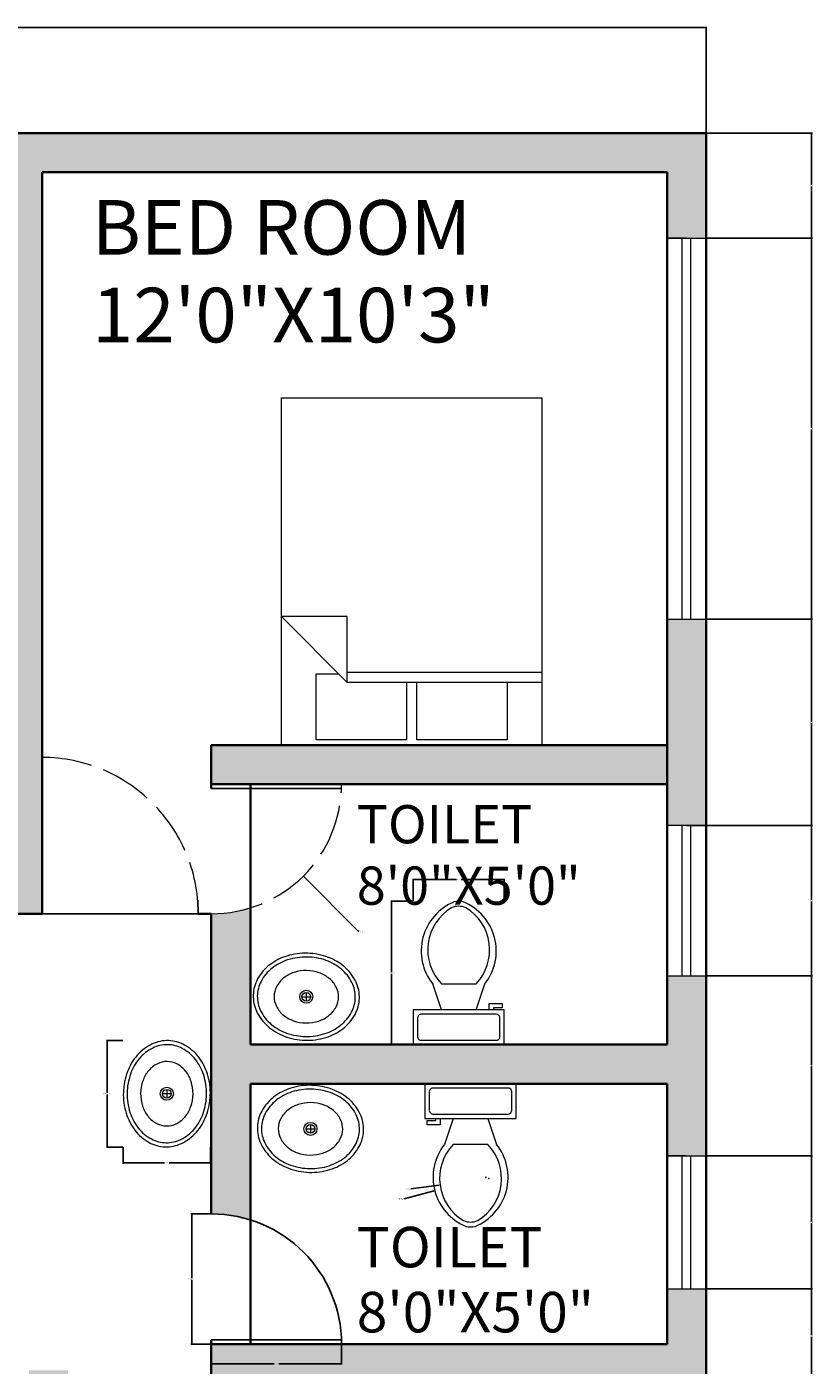
# Model space of a CAD drawing. Units: inches. Extents: x 582 to 1090, y 270 to 781.
# Tile 5 of 5: x 909 to 1090, y 461 to 769. Entities that reach past the tile are written whole.
import ezdxf

# ---------------------------------------------------------------- set-up
doc = ezdxf.new("R2010")
doc.units = ezdxf.units.IN
doc.header["$MEASUREMENT"] = 0
doc.linetypes.add('ACAD_ISO02W100', pattern=[15, 12, -3])
for name, color, linetype, lineweight in [('A-ANNO-DIMS', 2, 'Continuous', 18), ('A-AREA-IDEN', 7, 'Continuous', 25), ('A-DOOR', 3, 'Continuous', 25), ('A-DOOR-SWNG', 3, 'ACAD_ISO02W100', 13), ('A-FLOR-FIXT', 9, 'Continuous', 18), ('A-FURN', 8, 'Continuous', 18), ('A-GLAZ', 4, 'Continuous', 18), ('A-WALL', 7, 'Continuous', 35)]:
    doc.layers.add(name, color=color, linetype=linetype, lineweight=lineweight)
doc.layers.add('A-WALL-PATT', color=9, linetype='Continuous', lineweight=13, true_color=0xc7c8ca)
doc.styles.get("Standard").update_dxf_attribs({"font": 'arial.ttf'})
doc.dimstyles.get("Standard").update_dxf_attribs({"dimtxt": 0.18, "dimasz": 0.18, "dimexe": 0.18, "dimexo": 0.0625, "dimgap": 0.09, "dimtad": 0, "dimtih": 1, "dimtoh": 1, "dimdec": 0, "dimzin": 0, "dimdsep": 46, "dimlunit": 3, "dimtxsty": 'Standard', "dimcen": 0.09, "dimadec": 0, "dimazin": 0, "dimtfac": 1, "dimtdec": 0, "dimtofl": 0, "dimtmove": 0, "dimatfit": 3, "dimfxl": 1, "dimtolj": 1, "dimtzin": 0, "dimarcsym": 0})

# ---------------------------------------------------------------- blocks, each defined once
blk = doc.blocks.new('Toilet - top')
for p, q in [((9.5, -6), (9.5, -2)), ((-10, -8.5), (-8, -8.5)), ((-10, -9.5), (-10, -8.5)), ((-8, -8.5), (-8, -8)), ((-7, -8), (-7, -9.5)), ((-4, -8), (-6, -14)), ((4, -8), (6, -14)), ((-7, -9.5), (-10, -9.5)), ((4, -14), (-4, -14))]:
    blk.add_line(p, q)
blk.add_lwpolyline([(10.5, -8), (10.5, 0), (-10.5, 0), (-10.5, -8)], close=True)
for points in [[(-9.5, -2), (-9.5, -6)], [(8.5, -1), (-8.5, -1)], [(-8.5, -7), (8.5, -7)]]:
    blk.add_lwpolyline(points)
for centre, radius, start, end in [((-8.62, -1.88), 0.884, 81.8699, 188.1301), ((8.62, -1.88), 0.884, 351.8699, 98.1301), ((-8.62, -6.12), 0.884, 171.8699, 278.1301), ((8.62, -6.12), 0.884, 261.8699, 8.1301), ((3.52, -21.58), 12.17, 141.4691, 247.9714), ((4.2, -21.82), 11.33, 136.3677, 238.9468), ((-3.52, -21.58), 12.17, 292.0284, 38.5307), ((-4.2, -21.82), 11.33, 301.053, 43.6321), ((0, -27.88), 4, 245.7318, 294.2682), ((0, -29), 4, 254.8605, 285.1395)]:
    blk.add_arc(centre, radius, start, end)
blk = doc.blocks.new('Sink - Oval top')
for p, q in [((-1, 0), (1, 0)), ((0, 1), (0, -1))]:
    blk.add_line(p, q)
for points in [[(-12.23, 0.39, 0.117634), (-11.46, -3.36, 0.104469), (-8.88, -6.8, 0.090016), (-5.08, -9.07, 0.08192), (-0.32, -10.02, 0.08192), (4.49, -9.38, 0.090016), (8.42, -7.36, 0.104469), (11.22, -4.09, 0.117634), (12.23, -0.39, 0.117634), (11.46, 3.36, 0.104469), (8.88, 6.8, 0.090016), (5.08, 9.07, 0.08192), (0.32, 10.02, 0.08192), (-4.49, 9.38, 0.090016), (-8.42, 7.36, 0.104469), (-11.22, 4.09, 0.117634)], [(-11.29, 0.16, 0.118622), (-10.52, -3.25, 0.104678), (-8.07, -6.36, 0.089562), (-4.54, -8.37, 0.081185), (-0.13, -9.15, 0.081185), (4.3, -8.49, 0.089562), (7.89, -6.58, 0.104678), (10.42, -3.55, 0.118622), (11.29, -0.16, 0.118622), (10.52, 3.25, 0.104678), (8.07, 6.36, 0.089562), (4.54, 8.37, 0.081185), (0.13, 9.15, 0.081185), (-4.3, 8.49, 0.089562), (-7.89, 6.58, 0.104678), (-10.42, 3.55, 0.118622)], [(-7.42, 0.08, 0.118283), (-6.91, -2.17, 0.104607), (-5.29, -4.21, 0.089718), (-2.97, -5.53, 0.081436), (-0.07, -6.04, 0.081436), (2.84, -5.59, 0.089718), (5.2, -4.33, 0.104607), (6.86, -2.32, 0.118283), (7.42, -0.08, 0.118283), (6.91, 2.17, 0.104607), (5.29, 4.21, 0.089718), (2.97, 5.53, 0.081436), (0.07, 6.04, 0.081436), (-2.84, 5.59, 0.089718), (-5.2, 4.33, 0.104607), (-6.86, 2.32, 0.118283)]]:
    blk.add_lwpolyline(points, format="xyb", close=True)
for radius in [1.5, 1]:
    blk.add_circle((0, 0), radius)
blk = doc.blocks.new('Bed - Queen')
for p, q in [((0, -80.00003), (0, 0)), ((0, 0), (59.99999, 0)), ((59.99999, 0), (59.99999, -80.00003)), ((7.99999, -1.2), (28.79998, -1.2)), ((7.99999, -14.4), (7.99999, -1.2)), ((28.79998, -1.2), (28.79998, -14.4)), ((31.19999, -1.2), (51.99999, -1.2)), ((31.19999, -14.4), (31.19999, -1.2)), ((51.99999, -1.2), (51.99999, -16.4)), ((0, -14.4), (44.8, -14.4)), ((59.99999, -29.6), (44.8, -14.4)), ((44.8, -14.4), (44.8, -29.6)), ((44.8, -16.8), (0, -16.8)), ((51.99999, -16.4), (46.79936, -16.4)), ((44.8, -29.6), (59.99999, -29.6)), ((59.99999, -80.00003), (0, -80.00003))]:
    blk.add_line(p, q)
blk = doc.blocks.new('DOOR-SINGLE-30IN')
for p, q in [((29, 0), (29, 30)), ((30, 0), (30, 30))]:
    blk.add_line(p, q)
blk.add_arc((30, 0), 30, 90, 180)
blk = doc.blocks.new('*D12')
at = {"layer": 'A-ANNO-DIMS', "color": 0, "lineweight": -2, "transparency": 16777216}
for p, q in [((931.42, 535.41), (927.62, 535.41)), ((927.8, 535.23), (927.8, 523.32)), ((927.8, 511.04), (927.8, 522.96)), ((931.42, 510.86), (927.62, 510.86))]:
    blk.add_line(p, q, dxfattribs=at)
at = {"layer": 'A-ANNO-DIMS', "color": 0, "transparency": 16777216}
for points in [[(927.77, 535.23), (927.83, 535.23), (927.8, 535.41)], [(927.77, 511.04), (927.83, 511.04), (927.8, 510.86)]]:
    blk.add_solid(points, dxfattribs=at)
at = {"layer": 'Defpoints', "color": 0, "transparency": 16777216}
for p in [(931.49, 535.41), (927.8, 510.86), (931.49, 510.86)]:
    blk.add_point(p, dxfattribs=at)
at = {"layer": 'A-ANNO-DIMS', "color": 0, "transparency": 16777216, "insert": (927.8, 523.14), "char_height": 0.18, "attachment_point": 5}
blk.add_mtext('\\A1;BASIN 25 TYP.', dxfattribs=at)
blk = doc.blocks.new('*D13')
at = {"layer": 'A-ANNO-DIMS', "color": 0, "lineweight": -2, "transparency": 16777216}
for p, q in [((931.49, 510.8), (931.49, 507)), ((951.62, 510.8), (951.62, 507)), ((931.67, 507.18), (941.03, 507.18)), ((951.44, 507.18), (942.08, 507.18))]:
    blk.add_line(p, q, dxfattribs=at)
at = {"layer": 'A-ANNO-DIMS', "color": 0, "transparency": 16777216}
for points in [[(931.67, 507.21), (931.67, 507.15), (931.49, 507.18)], [(951.44, 507.21), (951.44, 507.15), (951.62, 507.18)]]:
    blk.add_solid(points, dxfattribs=at)
at = {"layer": 'Defpoints', "color": 0, "transparency": 16777216}
for p in [(931.49, 510.86), (951.62, 510.86), (951.62, 507.18)]:
    blk.add_point(p, dxfattribs=at)
at = {"layer": 'A-ANNO-DIMS', "color": 0, "transparency": 16777216, "insert": (941.56, 507.18), "char_height": 0.18, "attachment_point": 5}
blk.add_mtext('\\A1;20 TYP.', dxfattribs=at)
blk = doc.blocks.new('*D14')
at = {"layer": 'A-ANNO-DIMS', "color": 0, "lineweight": -2, "transparency": 16777216}
for p, q in [((998.24, 567.49), (993.17, 567.49)), ((993.35, 567.31), (993.35, 551.15)), ((993.35, 534.63), (993.35, 550.79)), ((998.24, 534.45), (993.17, 534.45))]:
    blk.add_line(p, q, dxfattribs=at)
at = {"layer": 'A-ANNO-DIMS', "color": 0, "transparency": 16777216}
for points in [[(993.32, 567.31), (993.38, 567.31), (993.35, 567.49)], [(993.32, 534.63), (993.38, 534.63), (993.35, 534.45)]]:
    blk.add_solid(points, dxfattribs=at)
at = {"layer": 'Defpoints', "color": 0, "transparency": 16777216}
for p in [(998.3, 567.49), (993.35, 534.45), (998.3, 534.45)]:
    blk.add_point(p, dxfattribs=at)
at = {"layer": 'A-ANNO-DIMS', "color": 0, "transparency": 16777216, "insert": (993.35, 550.97), "char_height": 0.18, "attachment_point": 5}
blk.add_mtext('\\A1;WC 33 TYP.', dxfattribs=at)
blk = doc.blocks.new('*D15')
at = {"layer": 'A-ANNO-DIMS', "color": 0, "lineweight": -2, "transparency": 16777216}
for p, q in [((998.3, 567.55), (998.3, 572.63)), ((998.48, 572.45), (1008.28, 572.45)), ((1019.12, 572.45), (1009.33, 572.45)), ((1019.3, 567.55), (1019.3, 572.63))]:
    blk.add_line(p, q, dxfattribs=at)
at = {"layer": 'A-ANNO-DIMS', "color": 0, "transparency": 16777216}
for points in [[(998.48, 572.48), (998.48, 572.42), (998.3, 572.45)], [(1019.12, 572.48), (1019.12, 572.42), (1019.3, 572.45)]]:
    blk.add_solid(points, dxfattribs=at)
at = {"layer": 'Defpoints', "color": 0, "transparency": 16777216}
for p in [(998.3, 572.45), (998.3, 567.49), (1019.3, 567.49)]:
    blk.add_point(p, dxfattribs=at)
at = {"layer": 'A-ANNO-DIMS', "color": 0, "transparency": 16777216, "insert": (1008.8, 572.45), "char_height": 0.18, "attachment_point": 5}
blk.add_mtext('\\A1;21 TYP.', dxfattribs=at)
blk = doc.blocks.new('*D28')
at = {"layer": 'A-ANNO-DIMS', "color": 0, "lineweight": -2, "transparency": 16777216}
for p, q in [((951.74, 495.45), (947.12, 495.45)), ((947.3, 495.27), (947.3, 480.63)), ((947.3, 465.63), (947.3, 480.26)), ((951.74, 465.45), (947.12, 465.45))]:
    blk.add_line(p, q, dxfattribs=at)
at = {"layer": 'A-ANNO-DIMS', "color": 0, "transparency": 16777216}
for points in [[(947.27, 495.27), (947.33, 495.27), (947.3, 495.45)], [(947.27, 465.63), (947.33, 465.63), (947.3, 465.45)]]:
    blk.add_solid(points, dxfattribs=at)
at = {"layer": 'Defpoints', "color": 0, "transparency": 16777216}
for p in [(951.8, 495.45), (947.3, 465.45), (951.8, 465.45)]:
    blk.add_point(p, dxfattribs=at)
at = {"layer": 'A-ANNO-DIMS', "color": 0, "transparency": 16777216, "insert": (947.3, 480.45), "char_height": 0.18, "attachment_point": 5}
blk.add_mtext('\\A1;DOOR 30 TYP.', dxfattribs=at)
blk = doc.blocks.new('*D29')
at = {"layer": 'A-ANNO-DIMS', "color": 0, "lineweight": -2, "transparency": 16777216}
for p, q in [((951.8, 465.38), (951.8, 460.77)), ((981.8, 465.38), (981.8, 460.77)), ((951.98, 460.95), (966.28, 460.95)), ((981.62, 460.95), (967.33, 460.95))]:
    blk.add_line(p, q, dxfattribs=at)
at = {"layer": 'A-ANNO-DIMS', "color": 0, "transparency": 16777216}
for points in [[(951.98, 460.98), (951.98, 460.92), (951.8, 460.95)], [(981.62, 460.98), (981.62, 460.92), (981.8, 460.95)]]:
    blk.add_solid(points, dxfattribs=at)
at = {"layer": 'Defpoints', "color": 0, "transparency": 16777216}
for p in [(951.8, 465.45), (981.8, 465.45), (981.8, 460.95)]:
    blk.add_point(p, dxfattribs=at)
at = {"layer": 'A-ANNO-DIMS', "color": 0, "transparency": 16777216, "insert": (966.8, 460.95), "char_height": 0.18, "attachment_point": 5}
blk.add_mtext('\\A1;30 TYP.', dxfattribs=at)
blk = doc.blocks.new('*D34')
at = {"layer": 'A-ANNO-DIMS', "color": 0, "lineweight": -2, "transparency": 16777216}
for p, q in [((606.8, 744.51), (606.8, 768.93)), ((606.98, 768.75), (836.01, 768.75)), ((1065.62, 768.75), (836.6, 768.75)), ((1065.8, 744.51), (1065.8, 768.93))]:
    blk.add_line(p, q, dxfattribs=at)
at = {"layer": 'A-ANNO-DIMS', "color": 0, "transparency": 16777216}
for points in [[(606.98, 768.78), (606.98, 768.72), (606.8, 768.75)], [(1065.62, 768.78), (1065.62, 768.72), (1065.8, 768.75)]]:
    blk.add_solid(points, dxfattribs=at)
at = {"layer": 'Defpoints', "color": 0, "transparency": 16777216}
for p in [(1065.8, 768.75), (606.8, 744.45), (1065.8, 744.45)]:
    blk.add_point(p, dxfattribs=at)
at = {"layer": 'A-ANNO-DIMS', "color": 0, "transparency": 16777216, "insert": (836.3, 768.75), "char_height": 0.18, "attachment_point": 5}
blk.add_mtext('\\A1;459', dxfattribs=at)
blk = doc.blocks.new('*D52')
at = {"layer": 'A-ANNO-DIMS', "color": 0, "lineweight": -2, "transparency": 16777216}
for p, q in [((1065.87, 744.45), (1090.28, 744.45)), ((1090.1, 744.27), (1090.1, 732.52)), ((1090.1, 720.42), (1090.1, 732.16)), ((1065.87, 720.24), (1090.28, 720.24))]:
    blk.add_line(p, q, dxfattribs=at)
at = {"layer": 'A-ANNO-DIMS', "color": 0, "transparency": 16777216}
for points in [[(1090.07, 744.27), (1090.13, 744.27), (1090.1, 744.45)], [(1090.07, 720.42), (1090.13, 720.42), (1090.1, 720.24)]]:
    blk.add_solid(points, dxfattribs=at)
at = {"layer": 'Defpoints', "color": 0, "transparency": 16777216}
for p in [(1065.8, 744.45), (1090.1, 744.45), (1065.8, 720.24)]:
    blk.add_point(p, dxfattribs=at)
at = {"layer": 'A-ANNO-DIMS', "color": 0, "transparency": 16777216, "insert": (1090.1, 732.34), "char_height": 0.18, "attachment_point": 5}
blk.add_mtext('\\A1;24.21', dxfattribs=at)
blk = doc.blocks.new('*D53')
at = {"layer": 'A-ANNO-DIMS', "color": 0, "lineweight": -2, "transparency": 16777216}
for p, q in [((1065.87, 720.24), (1090.28, 720.24)), ((1090.1, 720.06), (1090.1, 676.52)), ((1090.1, 632.62), (1090.1, 676.16)), ((1065.87, 632.44), (1090.28, 632.44))]:
    blk.add_line(p, q, dxfattribs=at)
at = {"layer": 'A-ANNO-DIMS', "color": 0, "transparency": 16777216}
for points in [[(1090.07, 720.06), (1090.13, 720.06), (1090.1, 720.24)], [(1090.07, 632.62), (1090.13, 632.62), (1090.1, 632.44)]]:
    blk.add_solid(points, dxfattribs=at)
at = {"layer": 'Defpoints', "color": 0, "transparency": 16777216}
for p in [(1065.8, 720.24), (1090.1, 720.24), (1065.8, 632.44)]:
    blk.add_point(p, dxfattribs=at)
at = {"layer": 'A-ANNO-DIMS', "color": 0, "transparency": 16777216, "insert": (1090.1, 676.34), "char_height": 0.18, "attachment_point": 5}
blk.add_mtext('\\A1;87.8', dxfattribs=at)
blk = doc.blocks.new('*D54')
at = {"layer": 'A-ANNO-DIMS', "color": 0, "lineweight": -2, "transparency": 16777216}
for p, q in [((1065.87, 632.44), (1090.28, 632.44)), ((1090.1, 632.26), (1090.1, 608.87)), ((1090.1, 585.11), (1090.1, 608.5)), ((1065.87, 584.93), (1090.28, 584.93))]:
    blk.add_line(p, q, dxfattribs=at)
at = {"layer": 'A-ANNO-DIMS', "color": 0, "transparency": 16777216}
for points in [[(1090.07, 632.26), (1090.13, 632.26), (1090.1, 632.44)], [(1090.07, 585.11), (1090.13, 585.11), (1090.1, 584.93)]]:
    blk.add_solid(points, dxfattribs=at)
at = {"layer": 'Defpoints', "color": 0, "transparency": 16777216}
for p in [(1065.8, 632.44), (1090.1, 632.44), (1065.8, 584.93)]:
    blk.add_point(p, dxfattribs=at)
at = {"layer": 'A-ANNO-DIMS', "color": 0, "transparency": 16777216, "insert": (1090.1, 608.69), "char_height": 0.18, "attachment_point": 5}
blk.add_mtext('\\A1;47.5', dxfattribs=at)
blk = doc.blocks.new('*D55')
at = {"layer": 'A-ANNO-DIMS', "color": 0, "lineweight": -2, "transparency": 16777216}
for p, q in [((1065.87, 584.93), (1090.28, 584.93)), ((1090.1, 584.75), (1090.1, 567.78)), ((1090.1, 550.44), (1090.1, 567.41)), ((1065.87, 550.26), (1090.28, 550.26))]:
    blk.add_line(p, q, dxfattribs=at)
at = {"layer": 'A-ANNO-DIMS', "color": 0, "transparency": 16777216}
for points in [[(1090.07, 584.75), (1090.13, 584.75), (1090.1, 584.93)], [(1090.07, 550.44), (1090.13, 550.44), (1090.1, 550.26)]]:
    blk.add_solid(points, dxfattribs=at)
at = {"layer": 'Defpoints', "color": 0, "transparency": 16777216}
for p in [(1065.8, 584.93), (1090.1, 584.93), (1065.8, 550.26)]:
    blk.add_point(p, dxfattribs=at)
at = {"layer": 'A-ANNO-DIMS', "color": 0, "transparency": 16777216, "insert": (1090.1, 567.6), "char_height": 0.18, "attachment_point": 5}
blk.add_mtext('\\A1;34.675', dxfattribs=at)
blk = doc.blocks.new('*D56')
at = {"layer": 'A-ANNO-DIMS', "color": 0, "lineweight": -2, "transparency": 16777216}
for p, q in [((1065.87, 550.26), (1090.28, 550.26)), ((1090.1, 550.08), (1090.1, 529.74)), ((1090.1, 509.04), (1090.1, 529.38)), ((1065.87, 508.86), (1090.28, 508.86))]:
    blk.add_line(p, q, dxfattribs=at)
at = {"layer": 'A-ANNO-DIMS', "color": 0, "transparency": 16777216}
for points in [[(1090.07, 550.08), (1090.13, 550.08), (1090.1, 550.26)], [(1090.07, 509.04), (1090.13, 509.04), (1090.1, 508.86)]]:
    blk.add_solid(points, dxfattribs=at)
at = {"layer": 'Defpoints', "color": 0, "transparency": 16777216}
for p in [(1065.8, 550.26), (1090.1, 550.26), (1065.8, 508.86)]:
    blk.add_point(p, dxfattribs=at)
at = {"layer": 'A-ANNO-DIMS', "color": 0, "transparency": 16777216, "insert": (1090.1, 529.56), "char_height": 0.18, "attachment_point": 5}
blk.add_mtext('\\A1;41.4', dxfattribs=at)
blk = doc.blocks.new('*D57')
at = {"layer": 'A-ANNO-DIMS', "color": 0, "lineweight": -2, "transparency": 16777216}
for p, q in [((1065.87, 508.86), (1090.28, 508.86)), ((1090.1, 508.68), (1090.1, 493.72)), ((1090.1, 478.39), (1090.1, 493.35)), ((1065.87, 478.21), (1090.28, 478.21))]:
    blk.add_line(p, q, dxfattribs=at)
at = {"layer": 'A-ANNO-DIMS', "color": 0, "transparency": 16777216}
for points in [[(1090.07, 508.68), (1090.13, 508.68), (1090.1, 508.86)], [(1090.07, 478.39), (1090.13, 478.39), (1090.1, 478.21)]]:
    blk.add_solid(points, dxfattribs=at)
at = {"layer": 'Defpoints', "color": 0, "transparency": 16777216}
for p in [(1065.8, 508.86), (1090.1, 508.86), (1065.8, 478.21)]:
    blk.add_point(p, dxfattribs=at)
at = {"layer": 'A-ANNO-DIMS', "color": 0, "transparency": 16777216, "insert": (1090.1, 493.54), "char_height": 0.18, "attachment_point": 5}
blk.add_mtext('\\A1;30.64', dxfattribs=at)
blk = doc.blocks.new('*D58')
at = {"layer": 'A-ANNO-DIMS', "color": 0, "lineweight": -2, "transparency": 16777216}
for p, q in [((1065.87, 478.21), (1090.28, 478.21)), ((1090.1, 478.03), (1090.1, 467.51)), ((1090.1, 456.63), (1090.1, 467.15)), ((1056.87, 456.45), (1090.28, 456.45))]:
    blk.add_line(p, q, dxfattribs=at)
at = {"layer": 'A-ANNO-DIMS', "color": 0, "transparency": 16777216}
for points in [[(1090.07, 478.03), (1090.13, 478.03), (1090.1, 478.21)], [(1090.07, 456.63), (1090.13, 456.63), (1090.1, 456.45)]]:
    blk.add_solid(points, dxfattribs=at)
at = {"layer": 'Defpoints', "color": 0, "transparency": 16777216}
for p in [(1065.8, 478.21), (1090.1, 478.21), (1056.8, 456.45)]:
    blk.add_point(p, dxfattribs=at)
at = {"layer": 'A-ANNO-DIMS', "color": 0, "transparency": 16777216, "insert": (1090.1, 467.33), "char_height": 0.18, "attachment_point": 5}
blk.add_mtext('\\A1;21.77', dxfattribs=at)
blk = doc.blocks.new('*D68')
at = {"layer": 'A-ANNO-DIMS', "color": 0, "lineweight": -2, "transparency": 16777216}
for p, q in [((951.88, 594.45), (952.06, 594.45)), ((951.97, 594.36), (951.97, 594.54)), ((985.63, 560.6), (973.14, 573.16)), ((985.81, 560.6), (985.63, 560.6))]:
    blk.add_line(p, q, dxfattribs=at)
at = {"layer": 'A-ANNO-DIMS', "color": 0, "transparency": 16777216}
blk.add_solid([(973.16, 573.18), (973.11, 573.14), (973.01, 573.29)], dxfattribs=at)
at = {"layer": 'Defpoints', "color": 0, "transparency": 16777216}
for p in [(951.97, 594.45), (973.01, 573.29)]:
    blk.add_point(p, dxfattribs=at)
at = {"layer": 'A-ANNO-DIMS', "color": 0, "transparency": 16777216, "insert": (986.29, 560.6), "char_height": 0.18, "attachment_point": 5}
blk.add_mtext('\\A1;R29.84', dxfattribs=at)
blk = doc.blocks.new('*D78')
at = {"layer": 'A-ANNO-DIMS', "color": 0, "lineweight": -2, "transparency": 16777216}
for p, q in [((1014.96, 503.87), (1015.14, 503.87)), ((1015.05, 503.78), (1015.05, 503.96)), ((996.22, 498.92), (1003.11, 500.73))]:
    blk.add_line(p, q, dxfattribs=at)
at = {"layer": 'A-ANNO-DIMS', "color": 0, "transparency": 16777216}
blk.add_solid([(1003.1, 500.76), (1003.11, 500.7), (1003.28, 500.77)], dxfattribs=at)
at = {"layer": 'Defpoints', "color": 0, "transparency": 16777216}
for p in [(1015.05, 503.87), (1003.28, 500.77)]:
    blk.add_point(p, dxfattribs=at)
at = {"layer": 'A-ANNO-DIMS', "color": 0, "transparency": 16777216, "insert": (995.54, 498.92), "char_height": 0.18, "attachment_point": 5}
blk.add_mtext('\\A1;6X R12.17', dxfattribs=at)
blk = doc.blocks.new('*D79')
at = {"layer": 'A-ANNO-DIMS', "color": 0, "lineweight": -2, "transparency": 16777216}
for p, q in [((1015.64, 503.63), (1015.82, 503.63)), ((1015.73, 503.54), (1015.73, 503.72)), ((997.76, 501.21), (1004.32, 502.1))]:
    blk.add_line(p, q, dxfattribs=at)
at = {"layer": 'A-ANNO-DIMS', "color": 0, "transparency": 16777216}
blk.add_solid([(1004.32, 502.12), (1004.33, 502.07), (1004.5, 502.12)], dxfattribs=at)
at = {"layer": 'Defpoints', "color": 0, "transparency": 16777216}
for p in [(1015.73, 503.63), (1004.5, 502.12)]:
    blk.add_point(p, dxfattribs=at)
at = {"layer": 'A-ANNO-DIMS', "color": 0, "transparency": 16777216, "insert": (997.09, 501.21), "char_height": 0.18, "attachment_point": 5}
blk.add_mtext('\\A1;6X R11.33', dxfattribs=at)

msp = doc.modelspace()

# ---------------------------------------------------------------- hatches: boundary and pattern name
at = {"layer": 'A-WALL-PATT'}
h = msp.add_hatch(color=256, dxfattribs=at)
h.dxf.hatch_style = 1
h.paths.add_polyline_path([(867.8047, 744.446), (765.8047, 744.446), (606.8047, 744.446), (606.8047, 711.9379), (615.8047, 711.9379), (615.8047, 735.446), (756.8047, 735.446), (756.8047, 585.446), (765.8047, 585.446), (765.8047, 735.446), (868.9478, 735.446, -0.06325422)])
h.paths.add_polyline_path([(1065.8047, 744.446), (912.8047, 744.446), (903.8047, 744.446), (903.8047, 708.446), (903.8047, 594.446), (903.8047, 564.6071), (912.8047, 564.6071), (912.8047, 600.6071), (912.8047, 735.446), (1056.8047, 735.446), (1056.8047, 720.2375), (1065.8047, 720.2375)])
h.paths.add_polyline_path([(1065.8047, 632.4383), (1056.8047, 632.4383), (1056.8047, 594.446), (1056.8047, 584.9343), (1065.8047, 584.9343), (1065.8047, 594.446)], flags=17)
h.paths.add_polyline_path([(1056.8047, 603.446), (951.8047, 603.446), (951.8047, 594.446), (1056.8047, 594.446)], flags=17)
h.paths.add_polyline_path([(1065.8047, 525.446), (1065.8047, 550.2593), (1056.8047, 550.2593), (1056.8047, 534.446), (960.8047, 534.446), (960.8047, 565.946, -0.07397332), (952.1262, 564.6071), (951.8047, 564.6071), (951.8047, 495.446, -0.07632083), (960.8047, 494.0641), (960.8047, 525.446), (1056.8047, 525.446), (1056.8047, 508.8565), (1065.8047, 508.8565)])
h.paths.add_polyline_path([(1065.8047, 478.2143), (1056.8047, 478.2143), (1056.8047, 465.446), (951.8047, 465.446), (951.8047, 456.446), (1056.8047, 456.446), (1056.8047, 420.446), (1065.8047, 420.446), (1065.8047, 456.446)])
h.paths.add_polyline_path([(1065.8047, 420.446), (1056.8047, 420.446), (1017.8047, 420.446), (1017.8047, 456.446), (1008.8047, 456.446), (1008.8047, 411.446), (1038.8047, 411.446), (1065.8047, 411.446)])
h.paths.add_polyline_path([(1065.8047, 411.446), (1056.8047, 411.446), (1056.8047, 327.446), (1065.8047, 327.446)])
h.paths.add_polyline_path([(1065.8047, 327.446), (1056.8047, 327.446), (1017.8047, 327.446), (1017.8047, 382.8278, -0.07632083), (1008.8047, 381.446), (1008.8047, 327.446), (983.7348, 327.446), (983.7348, 318.446), (1065.8047, 318.446)])
h.paths.add_polyline_path([(946.9624, 327.446), (918.8047, 327.446), (918.8047, 369.8742), (918.8047, 459.446), (909.8047, 459.446), (909.8047, 369.8742), (909.8047, 318.446), (946.9624, 318.446)])
h.paths.add_polyline_path([(918.8047, 318.446), (909.8047, 318.446), (909.8047, 303.4372), (765.8047, 303.4372), (765.8047, 327.446), (756.8047, 327.446), (756.8047, 294.4372), (918.8047, 294.4372)])
h.paths.add_polyline_path([(909.8047, 378.8742), (882.3477, 378.8742), (882.3477, 347.0959), (889.3299, 347.0959), (889.3299, 369.8742), (909.8047, 369.8742)])
h.paths.add_polyline_path([(779.4225, 378.8742), (765.8047, 378.8742), (765.8047, 369.8742), (779.4225, 369.8742)])
h.paths.add_polyline_path([(765.8047, 516.446), (756.8047, 516.446), (756.8047, 480.446), (756.8047, 336.446), (724.1731, 336.446), (724.1731, 327.446), (765.8047, 327.446), (765.8047, 369.8742), (765.8047, 378.8742)])
h.paths.add_polyline_path([(615.8047, 516.446), (606.8047, 516.446), (606.8047, 327.446), (637.062, 327.446), (637.062, 336.446), (615.8047, 336.446)])
h.paths.add_polyline_path([(615.8047, 631.6498), (606.8047, 631.6498), (606.8047, 585.446), (606.8047, 569.338), (615.8047, 569.338), (615.8047, 585.446), (615.8047, 594.446)])
h.paths.add_polyline_path([(721.9478, 594.446), (615.8047, 594.446), (615.8047, 585.446), (627.9505, 585.446, -0.03261849), (629.8936, 585.446), (710.8047, 585.446), (710.8047, 525.446), (675.3033, 525.446), (675.3033, 516.446), (719.8047, 516.446), (720.8047, 516.446), (720.8047, 525.446), (719.8047, 525.446), (719.8047, 585.446), (720.8047, 585.446, -0.06325422)])
h.paths.add_polyline_path([(646.6852, 525.446), (615.8047, 525.446), (615.8047, 516.446), (645.3033, 516.446, -0.07632083)])
h.paths.add_polyline_path([(615.8047, 525.446), (615.8047, 539.7667), (606.8047, 539.7667), (606.8047, 516.446), (615.8047, 516.446)])

# ---------------------------------------------------------------- linework, layer by layer
at = {"layer": 'A-DOOR'}
for p, q in [((912.8047, 564.6071), (912.8047, 600.6071)), ((951.8047, 594.446), (981.8047, 594.446)), ((951.8047, 594.446), (951.8047, 593.446)), ((951.8047, 593.446), (951.8047, 594.446)), ((951.8047, 593.446), (981.8047, 593.446)), ((948.8047, 564.6071), (948.6663, 567.7605)), ((912.8047, 564.6071), (948.8047, 564.6071)), ((951.8047, 465.446), (951.8047, 466.446))]:
    msp.add_line(p, q, dxfattribs=at)
at = {"layer": 'A-DOOR-SWNG'}
for centre, radius, start, end in [((912.8047, 564.6071), 36, 0, 90), ((951.9654, 594.446), 29.8393, 269.691354, 0)]:
    msp.add_arc(centre, radius, start, end, dxfattribs=at)
at = {"layer": 'A-GLAZ'}
for p, q in [((1061.3047, 720.2375), (1056.8047, 720.2375)), ((1056.8047, 720.2375), (1065.8047, 720.2375)), ((1060.3047, 632.4383), (1060.3047, 720.2375)), ((1062.3047, 632.4383), (1062.3047, 720.2375)), ((1056.8047, 632.4383), (1065.8047, 632.4383)), ((1065.8047, 584.9343), (1056.8047, 584.9343)), ((1060.3047, 550.2593), (1060.3047, 584.9343)), ((1061.3047, 584.9343), (1065.8047, 584.9343)), ((1062.3047, 550.2593), (1062.3047, 584.9343)), ((1056.8047, 550.2593), (1065.8047, 550.2593)), ((1061.3047, 508.8565), (1056.8047, 508.8565)), ((1056.8047, 508.8565), (1065.8047, 508.8565)), ((1060.3047, 478.2143), (1060.3047, 508.8565)), ((1062.3047, 478.2143), (1062.3047, 508.8565)), ((1056.8047, 478.2143), (1065.8047, 478.2143))]:
    msp.add_line(p, q, dxfattribs=at)
at = {"layer": 'A-WALL'}
for p, q in [((912.8047, 744.446), (765.8047, 744.446)), ((1065.8047, 744.446), (912.8047, 744.446)), ((1065.8047, 594.446), (1065.8047, 744.446)), ((912.8047, 594.446), (912.8047, 735.446)), ((912.8047, 735.446), (1056.8047, 735.446)), ((1056.8047, 735.446), (1056.8047, 594.446)), ((951.8047, 603.446), (1056.8047, 603.446)), ((951.8047, 593.446), (951.8047, 603.446)), ((912.8047, 564.6071), (912.8047, 594.446)), ((951.8047, 594.446), (1056.8047, 594.446)), ((960.8047, 534.446), (960.8047, 594.446)), ((1056.8047, 594.446), (1056.8047, 534.446)), ((1065.8047, 594.446), (1065.8047, 318.446)), ((903.8047, 564.6071), (912.8047, 564.6071)), ((951.8047, 564.6071), (948.8047, 564.6071)), ((951.8047, 534.446), (951.8047, 564.6071)), ((951.8047, 495.446), (951.8047, 564.6071)), ((1056.8047, 534.446), (960.8047, 534.446)), ((1056.8047, 525.446), (960.8047, 525.446)), ((960.8047, 465.446), (960.8047, 525.446)), ((1056.8047, 525.446), (1056.8047, 465.446)), ((1065.8047, 525.446), (1065.8047, 465.446)), ((951.8047, 456.446), (951.8047, 466.446)), ((1056.8047, 465.446), (951.8047, 465.446))]:
    msp.add_line(p, q, dxfattribs=at)

# ---------------------------------------------------------------- block references
at = {"layer": 'A-DOOR', "rotation": 269.9999999999998}
msp.add_blockref('DOOR-SINGLE-30IN', (951.8047, 495.4463), dxfattribs=at)
at = {"layer": 'A-FLOR-FIXT'}
for name, p, rotation in [('Toilet - top', (1008.8047, 534.446), 180), ('Sink - Oval top', (941.5552, 523.1387), 270)]:
    msp.add_blockref(name, p, dxfattribs=dict(at, rotation=rotation))
for name, p in [('Sink - Oval top', (973.693, 545.4778)), ('Sink - Oval top', (974.6475, 515.0452)), ('Toilet - top', (1011.5297, 525.446))]:
    msp.add_blockref(name, p, dxfattribs=at)
at = {"layer": 'A-FURN', "rotation": 180}
msp.add_blockref('Bed - Queen', (1027.9385, 603.446), dxfattribs=at)

# ---------------------------------------------------------------- texts
at = {"layer": 'A-ANNO-DIMS'}
for s, height, p in [('12\'0"X10\'3"', 12.580749, (924.3048, 696.216)), ('8\'0"X5\'0"', 8.80313, (985.3127, 566.675)), ('8\'0"X5\'0"', 9.32307, (985.3127, 468.1654))]:
    msp.add_text(s, height=height, dxfattribs=at).set_placement(p)
at = {"layer": 'A-AREA-IDEN'}
for s, height, p in [('BED ROOM', 12.58075, (924.3048, 716.4258)), ('TOILET', 8.80313, (985.3127, 580.8165)), ('TOILET', 9.32307, (985.3127, 483.1421))]:
    msp.add_text(s, height=height, dxfattribs=at).set_placement(p)

# ---------------------------------------------------------------- dimensions: what is measured, and where the dimension line sits
at = {"layer": 'A-ANNO-DIMS'}
dim = msp.add_linear_dim(base=(1065.8047, 768.746), p1=(606.8047, 744.446), p2=(1065.8047, 744.446), dimstyle='Standard', override={"dimdec": 0, "dimlfac": 1, "dimrnd": 0, "dimzin": 0, "dimdsep": 46, "dimlunit": 2}, dxfattribs=at)
dim.commit()
dim.dimension.update_dxf_attribs({"geometry": '*D34', "text_midpoint": (836.3047, 768.746)})
for base, p1, p2, override, picture, middle in [((1090.1047, 744.446), (1065.8047, 720.2375), (1065.8047, 744.446), {"dimdec": 2, "dimlfac": 1, "dimrnd": 0, "dimzin": 0, "dimdsep": 46, "dimlunit": 2}, '*D52', (1090.1047, 732.3417)), ((1090.1047, 720.2375), (1065.8047, 632.4383), (1065.8047, 720.2375), {"dimdec": 1, "dimlfac": 1, "dimrnd": 0, "dimzin": 0, "dimdsep": 46, "dimlunit": 2}, '*D53', (1090.1047, 676.3379)), ((1090.1047, 632.4383), (1065.8047, 584.9343), (1065.8047, 632.4383), {"dimdec": 1, "dimlfac": 1, "dimrnd": 0, "dimzin": 0, "dimdsep": 46, "dimlunit": 2}, '*D54', (1090.1047, 608.6863)), ((1090.1047, 584.9343), (1065.8047, 550.2593), (1065.8047, 584.9343), {"dimdec": 3, "dimlfac": 1, "dimrnd": 0, "dimzin": 0, "dimdsep": 46, "dimlunit": 2}, '*D55', (1090.1047, 567.5968)), ((1090.1047, 550.2593), (1065.8047, 508.8565), (1065.8047, 550.2593), {"dimdec": 1, "dimlfac": 1, "dimrnd": 0, "dimzin": 0, "dimdsep": 46, "dimlunit": 2}, '*D56', (1090.1047, 529.5579)), ((1090.1047, 508.8565), (1065.8047, 478.2143), (1065.8047, 508.8565), {"dimdec": 2, "dimlfac": 1, "dimrnd": 0, "dimzin": 0, "dimdsep": 46, "dimlunit": 2}, '*D57', (1090.1047, 493.5354)), ((1090.1047, 478.2143), (1056.8047, 456.446), (1065.8047, 478.2143), {"dimdec": 2, "dimlfac": 1, "dimrnd": 0, "dimzin": 0, "dimdsep": 46, "dimlunit": 2}, '*D58', (1090.1047, 467.3301))]:
    dim = msp.add_linear_dim(base=base, p1=p1, p2=p2, angle=90, dimstyle='Standard', override=override, dxfattribs=at)
    dim.commit()
    dim.dimension.update_dxf_attribs({"geometry": picture, "text_midpoint": middle})
dim = msp.add_radius_dim(center=(951.9654, 594.446), mpoint=(973.0082, 573.2898), dimstyle='Standard', override={"dimdec": 2, "dimlfac": 1, "dimrnd": 0, "dimzin": 0, "dimdsep": 46, "dimlunit": 2}, dxfattribs=at)
dim.commit()
dim.dimension.update_dxf_attribs({"geometry": '*D68', "text_midpoint": (986.2933, 560.5961), "dimtype": 164})
for base, p1, p2, angle, text, picture, middle in [((998.3047, 572.4491), (1019.3047, 567.4922), (998.3047, 567.4922), 180, '<> TYP.', '*D15', (1008.8047, 572.4491)), ((993.3477, 534.446), (998.3047, 567.4922), (998.3047, 534.446), 270, 'WC <> TYP.', '*D14', (993.3477, 550.9691)), ((927.8043, 510.8633), (931.4869, 535.4142), (931.4869, 510.8633), 270, 'BASIN <> TYP.', '*D12', (927.8043, 523.1387)), ((947.3047, 465.446), (951.8047, 495.446), (951.8047, 465.446), 270, 'DOOR <> TYP.', '*D28', (947.3047, 480.446))]:
    dim = msp.add_linear_dim(base=base, p1=p1, p2=p2, angle=angle, text=text, dimstyle='Standard', override={"dimdec": 0, "dimlfac": 1, "dimrnd": 0, "dimzin": 0, "dimdsep": 46, "dimlunit": 2}, dxfattribs=at)
    dim.commit()
    dim.dimension.update_dxf_attribs({"geometry": picture, "text_midpoint": middle})
for base, p1, p2, picture, middle in [((951.6235, 507.1806), (931.4869, 510.8633), (951.6235, 510.8633), '*D13', (941.5552, 507.1806)), ((981.8047, 460.946), (951.8047, 465.446), (981.8047, 465.446), '*D29', (966.8047, 460.946))]:
    dim = msp.add_linear_dim(base=base, p1=p1, p2=p2, text='<> TYP.', dimstyle='Standard', override={"dimdec": 0, "dimlfac": 1, "dimrnd": 0, "dimzin": 0, "dimdsep": 46, "dimlunit": 2}, dxfattribs=at)
    dim.commit()
    dim.dimension.update_dxf_attribs({"geometry": picture, "text_midpoint": middle})
for center, mpoint, picture, middle in [((1015.0492, 503.8655), (1003.2797, 500.7729), '*D78', (996.218, 498.9174)), ((1015.7296, 503.6286), (1004.5015, 502.1191), '*D79', (997.7646, 501.2134))]:
    dim = msp.add_radius_dim(center=center, mpoint=mpoint, text='6X <>', dimstyle='Standard', override={"dimdec": 2, "dimlfac": 1, "dimrnd": 0, "dimzin": 0, "dimdsep": 46, "dimlunit": 2}, dxfattribs=at)
    dim.commit()
    dim.dimension.update_dxf_attribs({"geometry": picture, "text_midpoint": middle, "dimtype": 164})

doc.saveas('drawing.dxf')
